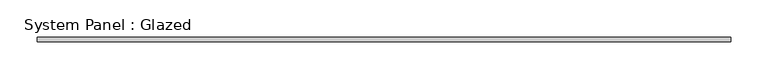
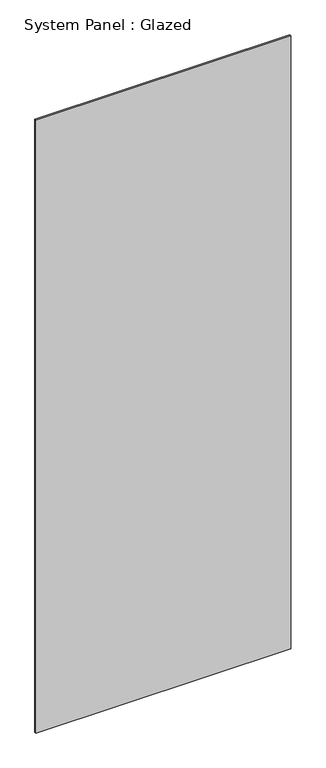
"""IFC4 building model written with IfcOpenShell, lengths in millimetres: plate geometry, System Panel : Glazed."""

from ifc_helpers import new_model, si_unit, origin, origin_with_axes, place, context, project, spatial, polyline, outline, extrude, source, transform, mapped, element, save


def system_panel_glazed_9bec98e5(model_context):
    return source(origin(), model_context, "Body", "SweptSolid", [
        extrude(outline(polyline([(462.5, 34.0), (-462.5, 34.0), (-462.5, 40.0), (462.5, 40.0), (462.5, 34.0)])), origin_with_axes(), (0.0, 0.0, 1.0), 2350.0),
    ])


if __name__ == "__main__":
    model = new_model("IFC4")
    model_context = context("Model", 3, world=origin())
    ifc_project = project(units=[si_unit("LENGTHUNIT", "METRE", prefix="MILLI")], contexts=[model_context])
    site = spatial("IfcSite", under=ifc_project)
    building = spatial("IfcBuilding", under=site)
    placement = place(None, origin())
    system_panel_glazed_shape = system_panel_glazed_9bec98e5(model_context)
    element("IfcPlate", 1, ObjectType="System Panel : Glazed", at=placement, inside=building, context=model_context, shape_type="MappedRepresentation", body=[
        mapped(system_panel_glazed_shape, transform((0.0, 0.0, 0.0), x_axis=(1.0, 0.0, 0.0), y_axis=(0.0, 1.0, 0.0), z_axis=(0.0, 0.0, 1.0))),
    ])
    save(model, "model.ifc")

# Revit data of these elements
# Type "System Panel : Glazed"
#   Construction Type Id = "GSP4R"
#   Analytic Construction = "1/8 in Pilkington single glazing"
#   Visual Light Transmittance = 0.9
#   Solar Heat Gain Coefficient = 0.86
#   Heat Transfer Coefficient (U) = 6.7069 W/(m²·K)
#   Define Thermal Properties by = 1
# Element 1 (IfcPlate, "System Panel : Glazed")
#   Materials on its faces: "Default New Material(6)"
# Materials
#   "Default New Material(6)": class "Generic", colour RGB 191 25 25, transparency 0.9, Cost = 0
